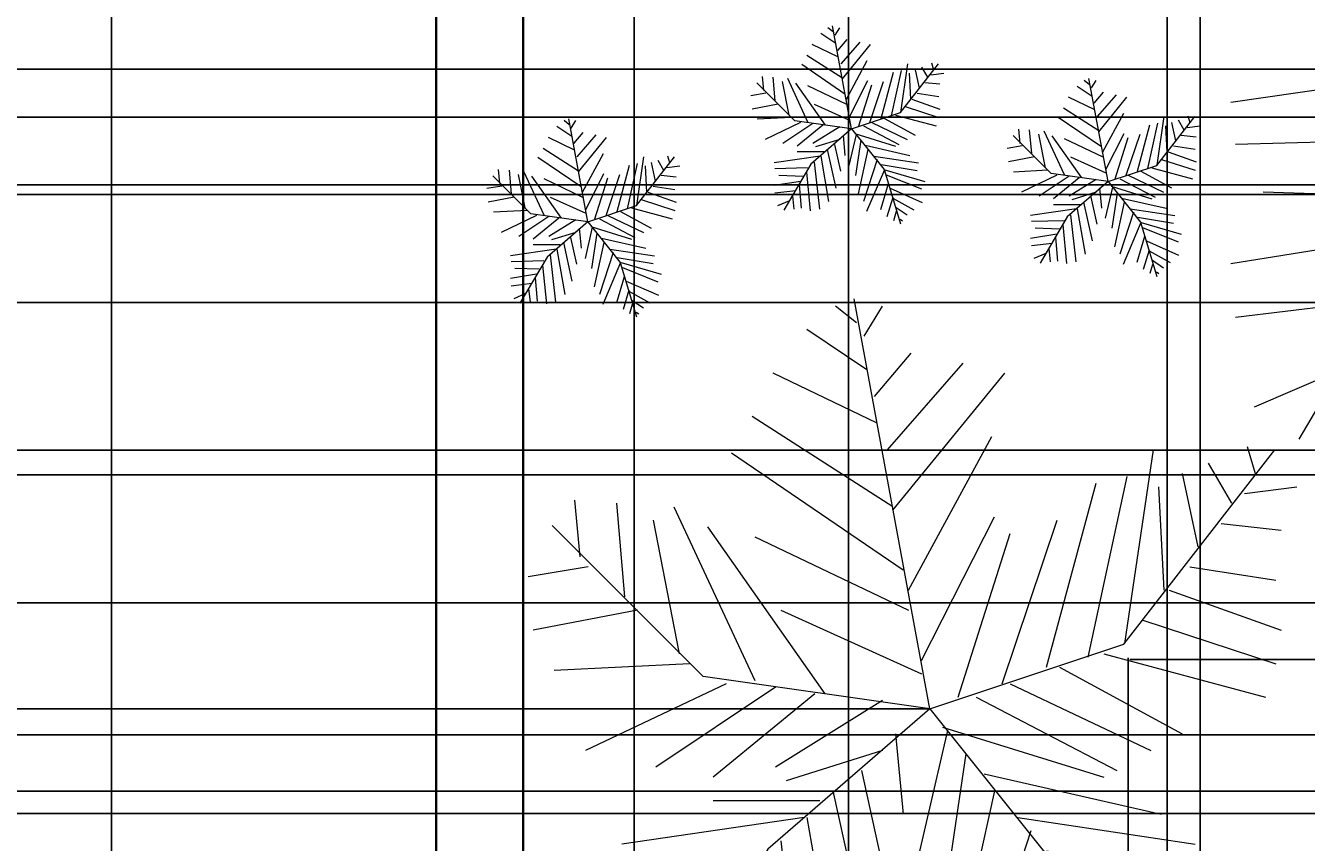
# Model space of a CAD drawing. Units: inches. Extents: x 818 to 1898, y 976 to 2364.
# Tile 58 of 96: x 950 to 1083, y 1873 to 1958. Entities that reach past the tile are written whole.
import ezdxf

# ---------------------------------------------------------------- set-up
doc = ezdxf.new("R2010")
doc.units = ezdxf.units.IN
doc.header["$LTSCALE"] = 5
doc.header["$MEASUREMENT"] = 0
for name, color, linetype, lineweight in [('A-ANNO-DIMS', 2, 'Continuous', 18), ('C-PROP', 7, 'Continuous', 35), ('L-PLNT-BEDS', 94, 'Continuous', 18)]:
    doc.layers.add(name, color=color, linetype=linetype, lineweight=lineweight)
doc.layers.add('L-PLNT', color=116, linetype='Continuous', lineweight=13, true_color=0x136734)
doc.styles.get("Standard").update_dxf_attribs({"font": 'arial.ttf'})
doc.dimstyles.get("Standard").update_dxf_attribs({"dimtxt": 0.18, "dimasz": 0.18, "dimexe": 0.18, "dimexo": 0.0625, "dimgap": 0.09, "dimtad": 0, "dimtih": 1, "dimtoh": 1, "dimdec": 4, "dimzin": 0, "dimdsep": 46, "dimtxsty": 'Standard', "dimcen": 0.09, "dimadec": 0, "dimazin": 0, "dimtfac": 1, "dimtdec": 4, "dimtofl": 0, "dimtmove": 0, "dimatfit": 3, "dimfxl": 1, "dimtolj": 1, "dimtzin": 0, "dimarcsym": 0})

# ---------------------------------------------------------------- blocks, each defined once
blk = doc.blocks.new('SHRUB-ACCENT')
for p, q in [((8.53, 19.84), (7.99, 20.28)), ((10.44, 9.82), (8.47, 20.47)), ((8.74, 19.5), (9.21, 20.28)), ((8.8, 18.63), (7.25, 19.67)), ((9.01, 17.93), (9.96, 19.06)), ((9.35, 16.54), (11.31, 18.8)), ((9.48, 15.07), (5.82, 17.41)), ((9.08, 17.24), (6.37, 18.54)), ((9.48, 14.98), (12.39, 18.54)), ((9.75, 13.42), (5.28, 16.46)), ((9.89, 12.9), (12.06, 16.89)), ((15.49, 11.5), (19.41, 16.55)), ((15.51, 11.51), (16.25, 16.54)), ((17, 15.94), (17.41, 14.03)), ((17.68, 16.2), (18.29, 15.16)), ((18.69, 16.63), (18.9, 15.94)), ((4.55, 10.66), (0.62, 14.58)), ((1.35, 13.77), (1.22, 15.24)), ((2.3, 15.16), (2.51, 12.72)), ((3.25, 14.72), (3.93, 11.25)), ((3.79, 15.07), (5.89, 10.55)), ((10.23, 11.07), (12.12, 14.81)), ((12.33, 10.47), (13.75, 14.72)), ((13.48, 10.9), (14.76, 15.68)), ((14.56, 11.16), (15.58, 15.85)), ((16.39, 15.59), (16.53, 12.9)), ((18.02, 14.63), (19.57, 14.46)), ((18.62, 15.42), (19.98, 15.59)), ((1.56, 13.51), (0, 13.25)), ((7.72, 10.21), (4.67, 14.55)), ((5.89, 14.29), (9.89, 12.38)), ((11.17, 10.12), (12.53, 14.37)), ((17.2, 13.51), (19.44, 13.16)), ((2.84, 12.38), (0.14, 11.86)), ((6.57, 12.38), (10.23, 10.73)), ((15.98, 12.12), (19.44, 10.99)), ((16.66, 12.9), (19.57, 11.86)), ((4.2, 10.99), (0.68, 10.81)), ((10.44, 9.82), (4.55, 10.66)), ((10.44, 9.82), (15.49, 11.5)), ((13.82, 10.9), (17, 9.16)), ((14.97, 11.25), (19.17, 10.12)), ((5.15, 10.47), (1.49, 8.73)), ((6.43, 10.38), (3.32, 8.3)), ((7.45, 10.21), (4.81, 8.04)), ((10.44, 9.82), (6.23, 6.17)), ((9.21, 10.03), (6.43, 8.3)), ((10.44, 9.82), (13.8, 5.61)), ((10.77, 9.34), (14.97, 8.04)), ((11.65, 10.12), (15.31, 8.21)), ((12.53, 10.47), (16.19, 8.73)), ((9.21, 8.73), (6.7, 7.95)), ((8.67, 8.21), (9.28, 5.43)), ((9.55, 9.16), (9.75, 7.08)), ((10.9, 9.25), (10.16, 6.04)), ((11.38, 8.64), (10.84, 5)), ((11.85, 8.12), (16.46, 7.08)), ((7.18, 6.99), (2.44, 6.3)), ((7.59, 7.43), (4.81, 7.43)), ((7.25, 6.99), (8.06, 2.31)), ((7.92, 7.69), (8.8, 3.69)), ((12.12, 7.69), (11.11, 3.09)), ((13.07, 6.65), (11.65, 2.31)), ((12.73, 6.99), (17.34, 6.3)), ((5.89, 5.78), (2.51, 5.69)), ((6.23, 6.17), (3.43, 1.4)), ((5.76, 5.34), (6.16, 1.35)), ((6.57, 6.39), (7.11, 1.52)), ((13.82, 5.6), (11.99, 1.26)), ((13.48, 6.13), (17.2, 5.52)), ((13.8, 5.61), (15.49, 0)), ((13.88, 5.6), (18.02, 4.39)), ((5.15, 4.39), (2.44, 3.95)), ((5.42, 4.91), (2.91, 5)), ((5.01, 4.04), (5.21, 1.61)), ((14.22, 4.13), (13.41, 1.44)), ((14.02, 5.08), (17.68, 3.61)), ((4.67, 3.43), (2.51, 3.17)), ((4.33, 2.91), (4.47, 1.52)), ((14.7, 2.74), (14.09, 0.74)), ((14.43, 3.69), (17.74, 2.22)), ((14.7, 2.65), (16.86, 1.44)), ((4, 2.39), (2.78, 1.87)), ((15.04, 1.7), (16.19, 0.92)), ((15.04, 1.26), (14.76, 0.31)), ((15.44, 0.48), (15.71, 0.31))]:
    blk.add_line(p, q)
blk = doc.blocks.new('PALM-BORDER')
for p, q in [((41.53, 39.05), (33.72, 81.45)), ((33.95, 78.95), (31.8, 80.68)), ((34.76, 77.57), (36.65, 80.68)), ((35.03, 74.11), (28.83, 78.26)), ((35.84, 71.35), (39.61, 75.84)), ((37.18, 65.82), (45, 74.8)), ((36.11, 68.59), (25.33, 73.77)), ((37.72, 59.6), (49.31, 73.77)), ((37.72, 59.95), (23.17, 69.28)), ((39.34, 51.31), (47.96, 67.2)), ((38.8, 53.39), (21.02, 65.48)), ((61.61, 45.75), (77.23, 65.83)), ((61.71, 45.79), (64.67, 65.82)), ((74.37, 66.17), (75.18, 63.4)), ((70.33, 64.44), (72.75, 60.3)), ((53.62, 43.37), (58.74, 62.37)), ((57.93, 44.41), (61.97, 63.06)), ((67.63, 63.4), (69.25, 55.81)), ((65.21, 62.02), (65.75, 51.31)), ((74.1, 61.33), (79.49, 62.02)), ((5.39, 54.77), (4.85, 60.64)), ((9.16, 60.3), (9.97, 50.62)), ((15.09, 59.95), (23.44, 41.99)), ((12.93, 58.57), (15.63, 44.75)), ((40.69, 44.06), (48.23, 58.91)), ((49.04, 41.64), (54.7, 58.57)), ((18.1, 42.4), (2.48, 58.02)), ((30.72, 40.61), (18.59, 57.88)), ((44.46, 40.26), (49.85, 57.19)), ((71.68, 58.22), (77.87, 57.53)), ((23.44, 56.84), (39.34, 49.24)), ((6.2, 53.73), (0, 52.7)), ((68.44, 53.73), (77.33, 52.35)), ((66.29, 51.31), (77.87, 47.17)), ((11.32, 49.24), (0.54, 47.17)), ((26.14, 49.24), (40.69, 42.68)), ((63.59, 48.21), (77.33, 43.71)), ((41.53, 39.05), (61.61, 45.75)), ((16.71, 43.71), (2.69, 43.02)), ((59.55, 44.75), (76.26, 40.26)), ((41.53, 39.05), (18.1, 42.4)), ((54.97, 43.37), (67.63, 36.46)), ((20.48, 41.64), (5.93, 34.73)), ((25.6, 41.3), (13.2, 33.01)), ((49.85, 41.64), (64.4, 34.73)), ((29.64, 40.61), (19.13, 31.97)), ((36.65, 39.91), (25.6, 33.01)), ((46.35, 40.26), (60.9, 32.66)), ((41.53, 39.05), (24.79, 24.55)), ((41.53, 39.05), (54.92, 22.32)), ((42.84, 37.15), (59.55, 31.97)), ((37.99, 36.46), (38.8, 28.17)), ((43.38, 36.81), (40.42, 24.02)), ((36.65, 34.73), (26.68, 31.62)), ((45.27, 34.39), (43.11, 19.88)), ((34.49, 32.66), (36.92, 21.61)), ((47.15, 32.32), (65.48, 28.17)), ((31.53, 30.59), (35.03, 14.7)), ((48.23, 30.59), (44.19, 12.28)), ((30.18, 29.55), (19.13, 29.55)), ((28.56, 27.82), (9.7, 25.06)), ((28.83, 27.82), (32.07, 9.17)), ((50.66, 27.82), (68.98, 25.06)), ((26.14, 25.41), (28.29, 6.06)), ((52, 26.44), (46.35, 9.17)), ((24.79, 24.55), (13.63, 5.58)), ((53.62, 24.37), (68.44, 21.95)), ((23.44, 22.99), (9.97, 22.64)), ((22.9, 21.26), (24.52, 5.37)), ((54.97, 22.3), (47.69, 5.02)), ((54.92, 22.32), (61.61, 0)), ((55.24, 22.3), (71.68, 17.46)), ((21.56, 19.53), (11.59, 19.88)), ((55.78, 20.22), (70.33, 14.35)), ((20.48, 17.46), (9.7, 15.73)), ((19.94, 16.08), (20.75, 6.41)), ((56.59, 16.42), (53.35, 5.72)), ((57.39, 14.7), (70.6, 8.83)), ((18.59, 13.66), (9.97, 12.62)), ((17.24, 11.59), (17.78, 6.06)), ((58.47, 10.9), (56.05, 2.95)), ((15.9, 9.52), (11.05, 7.44)), ((58.47, 10.55), (67.09, 5.72)), ((59.82, 6.75), (64.4, 3.64)), ((59.82, 5.02), (58.74, 1.22)), ((61.44, 1.92), (62.51, 1.22))]:
    blk.add_line(p, q)
blk = doc.blocks.new('PALM-DECK')
for p, q in [((51.03, 49.71), (17.33, 44.77)), ((44.29, 43.85), (24.36, 9.97)), ((41.88, 41.07), (17.81, 40.45)), ((38.51, 34.9), (20.7, 35.52)), ((36.59, 31.2), (17.33, 28.11)), ((33.22, 24.41), (17.81, 22.55)), ((28.4, 17), (19.74, 13.3))]:
    blk.add_line(p, q)
blk = doc.blocks.new('*D29')
at = {"layer": 'A-ANNO-DIMS', "color": 0, "lineweight": -2, "ltscale": 5, "transparency": 16777216}
for p, q in [((1064.31, 1870.24), (1064.31, 1892.19)), ((1064.49, 1892.01), (1134.73, 1892.01)), ((1206.15, 1892.01), (1135.91, 1892.01)), ((1206.33, 1870.24), (1206.33, 1892.19))]:
    blk.add_line(p, q, dxfattribs=at)
at = {"layer": 'A-ANNO-DIMS', "color": 0, "ltscale": 5, "transparency": 16777216}
for points in [[(1064.49, 1892.04), (1064.49, 1891.98), (1064.31, 1892.01)], [(1206.15, 1892.04), (1206.15, 1891.98), (1206.33, 1892.01)]]:
    blk.add_solid(points, dxfattribs=at)
at = {"layer": 'Defpoints', "color": 0, "ltscale": 5, "transparency": 16777216}
for p in [(1206.33, 1892.01), (1064.31, 1870.18), (1206.33, 1870.18)]:
    blk.add_point(p, dxfattribs=at)
at = {"layer": 'A-ANNO-DIMS', "color": 0, "ltscale": 5, "transparency": 16777216, "insert": (1135.32, 1892.01), "char_height": 0.18, "attachment_point": 5}
blk.add_mtext('\\A1;142 TYP.', dxfattribs=at)
blk = doc.blocks.new('*D59')
at = {"layer": 'A-ANNO-DIMS', "color": 0, "lineweight": -2, "ltscale": 5, "transparency": 16777216}
for p, q in [((1251.64, 2300.39), (818.03, 2300.39)), ((818.21, 2300.21), (818.21, 1669.95)), ((818.21, 1039.32), (818.21, 1669.59)), ((896.05, 1039.14), (818.03, 1039.14))]:
    blk.add_line(p, q, dxfattribs=at)
at = {"layer": 'A-ANNO-DIMS', "color": 0, "ltscale": 5, "transparency": 16777216}
for points in [[(818.18, 2300.21), (818.24, 2300.21), (818.21, 2300.39)], [(818.18, 1039.32), (818.24, 1039.32), (818.21, 1039.14)]]:
    blk.add_solid(points, dxfattribs=at)
at = {"layer": 'Defpoints', "color": 0, "ltscale": 5, "transparency": 16777216}
for p in [(818.21, 2300.39), (1251.71, 2300.39), (896.11, 1039.14)]:
    blk.add_point(p, dxfattribs=at)
at = {"layer": 'A-ANNO-DIMS', "color": 0, "ltscale": 5, "transparency": 16777216, "insert": (818.21, 1669.77), "char_height": 0.18, "attachment_point": 5}
blk.add_mtext('\\A1;1261.2', dxfattribs=at)
blk = doc.blocks.new('*D60')
at = {"layer": 'A-ANNO-DIMS', "color": 0, "lineweight": -2, "ltscale": 5, "transparency": 16777216}
for p, q in [((992.66, 2294.22), (818.03, 2294.22)), ((818.21, 2294.04), (818.21, 1748.77)), ((818.21, 1203.14), (818.21, 1748.41)), ((992.66, 1202.96), (818.03, 1202.96))]:
    blk.add_line(p, q, dxfattribs=at)
at = {"layer": 'A-ANNO-DIMS', "color": 0, "ltscale": 5, "transparency": 16777216}
for points in [[(818.18, 2294.04), (818.24, 2294.04), (818.21, 2294.22)], [(818.18, 1203.14), (818.24, 1203.14), (818.21, 1202.96)]]:
    blk.add_solid(points, dxfattribs=at)
at = {"layer": 'Defpoints', "color": 0, "ltscale": 5, "transparency": 16777216}
for p in [(818.21, 2294.22), (992.73, 2294.22), (992.73, 1202.96)]:
    blk.add_point(p, dxfattribs=at)
at = {"layer": 'A-ANNO-DIMS', "color": 0, "ltscale": 5, "transparency": 16777216, "insert": (818.21, 1748.59), "char_height": 0.18, "attachment_point": 5}
blk.add_mtext('\\A1;1091.3', dxfattribs=at)
blk = doc.blocks.new('*D61')
at = {"layer": 'A-ANNO-DIMS', "color": 0, "lineweight": -2, "ltscale": 5, "transparency": 16777216}
for p, q in [((1071.73, 1203.03), (1071.73, 2363.87)), ((1071.91, 2363.69), (1250.94, 2363.69)), ((1430.55, 2363.69), (1251.51, 2363.69)), ((1430.73, 1203.03), (1430.73, 2363.87))]:
    blk.add_line(p, q, dxfattribs=at)
at = {"layer": 'A-ANNO-DIMS', "color": 0, "ltscale": 5, "transparency": 16777216}
for points in [[(1071.91, 2363.72), (1071.91, 2363.66), (1071.73, 2363.69)], [(1430.55, 2363.72), (1430.55, 2363.66), (1430.73, 2363.69)]]:
    blk.add_solid(points, dxfattribs=at)
at = {"layer": 'Defpoints', "color": 0, "ltscale": 5, "transparency": 16777216}
for p in [(1430.73, 2363.69), (1071.73, 1202.96), (1430.73, 1202.96)]:
    blk.add_point(p, dxfattribs=at)
at = {"layer": 'A-ANNO-DIMS', "color": 0, "ltscale": 5, "transparency": 16777216, "insert": (1251.23, 2363.69), "char_height": 0.18, "attachment_point": 5}
blk.add_mtext('\\A1;359', dxfattribs=at)
blk = doc.blocks.new('*D74')
at = {"layer": 'A-ANNO-DIMS', "color": 0, "lineweight": -2, "ltscale": 5, "transparency": 16777216}
for p, q in [((1590.66, 1940.08), (818.03, 1940.08)), ((818.21, 1939.9), (818.21, 1925.76)), ((818.21, 1911.26), (818.21, 1925.4)), ((1590.66, 1911.08), (818.03, 1911.08))]:
    blk.add_line(p, q, dxfattribs=at)
at = {"layer": 'A-ANNO-DIMS', "color": 0, "ltscale": 5, "transparency": 16777216}
for points in [[(818.18, 1939.9), (818.24, 1939.9), (818.21, 1940.08)], [(818.18, 1911.26), (818.24, 1911.26), (818.21, 1911.08)]]:
    blk.add_solid(points, dxfattribs=at)
at = {"layer": 'Defpoints', "color": 0, "ltscale": 5, "transparency": 16777216}
for p in [(818.21, 1940.08), (1590.73, 1940.08), (1590.73, 1911.08)]:
    blk.add_point(p, dxfattribs=at)
at = {"layer": 'A-ANNO-DIMS', "color": 0, "ltscale": 5, "transparency": 16777216, "insert": (818.21, 1925.58), "char_height": 0.18, "attachment_point": 5}
blk.add_mtext('\\A1;29', dxfattribs=at)
blk = doc.blocks.new('*D79')
at = {"layer": 'A-ANNO-DIMS', "color": 0, "lineweight": -2, "ltscale": 5, "transparency": 16777216}
for p, q in [((992.73, 1203.03), (992.73, 2363.87)), ((992.91, 2363.69), (1032.01, 2363.69)), ((1071.55, 2363.69), (1032.44, 2363.69)), ((1071.73, 1203.03), (1071.73, 2363.87))]:
    blk.add_line(p, q, dxfattribs=at)
at = {"layer": 'A-ANNO-DIMS', "color": 0, "ltscale": 5, "transparency": 16777216}
for points in [[(992.91, 2363.72), (992.91, 2363.66), (992.73, 2363.69)], [(1071.55, 2363.72), (1071.55, 2363.66), (1071.73, 2363.69)]]:
    blk.add_solid(points, dxfattribs=at)
at = {"layer": 'Defpoints', "color": 0, "ltscale": 5, "transparency": 16777216}
for p in [(1071.73, 2363.69), (992.73, 1202.96), (1071.73, 1202.96)]:
    blk.add_point(p, dxfattribs=at)
at = {"layer": 'A-ANNO-DIMS', "color": 0, "ltscale": 5, "transparency": 16777216, "insert": (1032.23, 2363.69), "char_height": 0.18, "attachment_point": 5}
blk.add_mtext('\\A1;79', dxfattribs=at)
blk = doc.blocks.new('*D90')
at = {"layer": 'A-ANNO-DIMS', "color": 0, "lineweight": -2, "ltscale": 5, "transparency": 16777216}
for p, q in [((904.95, 1071.12), (904.95, 2363.87)), ((905.13, 2363.69), (931.67, 2363.69)), ((958.99, 2363.69), (932.45, 2363.69)), ((959.17, 1071.12), (959.17, 2363.87))]:
    blk.add_line(p, q, dxfattribs=at)
at = {"layer": 'A-ANNO-DIMS', "color": 0, "ltscale": 5, "transparency": 16777216}
for points in [[(905.13, 2363.72), (905.13, 2363.66), (904.95, 2363.69)], [(958.99, 2363.72), (958.99, 2363.66), (959.17, 2363.69)]]:
    blk.add_solid(points, dxfattribs=at)
at = {"layer": 'Defpoints', "color": 0, "ltscale": 5, "transparency": 16777216}
for p in [(959.17, 2363.69), (904.95, 1071.06), (959.17, 1071.06)]:
    blk.add_point(p, dxfattribs=at)
at = {"layer": 'A-ANNO-DIMS', "color": 0, "ltscale": 5, "transparency": 16777216, "insert": (932.06, 2363.69), "char_height": 0.18, "attachment_point": 5}
blk.add_mtext('\\A1;54.22', dxfattribs=at)
blk = doc.blocks.new('*D91')
at = {"layer": 'A-ANNO-DIMS', "color": 0, "lineweight": -2, "ltscale": 5, "transparency": 16777216}
for p, q in [((959.17, 1071.12), (959.17, 2363.87)), ((959.35, 2363.69), (985.8, 2363.69)), ((1013.04, 2363.69), (986.59, 2363.69)), ((1013.22, 1071.12), (1013.22, 2363.87))]:
    blk.add_line(p, q, dxfattribs=at)
at = {"layer": 'A-ANNO-DIMS', "color": 0, "ltscale": 5, "transparency": 16777216}
for points in [[(959.35, 2363.72), (959.35, 2363.66), (959.17, 2363.69)], [(1013.04, 2363.72), (1013.04, 2363.66), (1013.22, 2363.69)]]:
    blk.add_solid(points, dxfattribs=at)
at = {"layer": 'Defpoints', "color": 0, "ltscale": 5, "transparency": 16777216}
for p in [(1013.22, 2363.69), (959.17, 1071.06), (1013.22, 1071.06)]:
    blk.add_point(p, dxfattribs=at)
at = {"layer": 'A-ANNO-DIMS', "color": 0, "ltscale": 5, "transparency": 16777216, "insert": (986.2, 2363.69), "char_height": 0.18, "attachment_point": 5}
blk.add_mtext('\\A1;54.04', dxfattribs=at)
blk = doc.blocks.new('*D92')
at = {"layer": 'A-ANNO-DIMS', "color": 0, "lineweight": -2, "ltscale": 5, "transparency": 16777216}
for p, q in [((1013.22, 1071.12), (1013.22, 2363.87)), ((1013.4, 2363.69), (1040.38, 2363.69)), ((1068.16, 2363.69), (1041.17, 2363.69)), ((1068.34, 1071.12), (1068.34, 2363.87))]:
    blk.add_line(p, q, dxfattribs=at)
at = {"layer": 'A-ANNO-DIMS', "color": 0, "ltscale": 5, "transparency": 16777216}
for points in [[(1013.4, 2363.72), (1013.4, 2363.66), (1013.22, 2363.69)], [(1068.16, 2363.72), (1068.16, 2363.66), (1068.34, 2363.69)]]:
    blk.add_solid(points, dxfattribs=at)
at = {"layer": 'Defpoints', "color": 0, "ltscale": 5, "transparency": 16777216}
for p in [(1068.34, 2363.69), (1013.22, 1071.06), (1068.34, 1071.06)]:
    blk.add_point(p, dxfattribs=at)
at = {"layer": 'A-ANNO-DIMS', "color": 0, "ltscale": 5, "transparency": 16777216, "insert": (1040.78, 2363.69), "char_height": 0.18, "attachment_point": 5}
blk.add_mtext('\\A1;55.12', dxfattribs=at)
blk = doc.blocks.new('*D93')
at = {"layer": 'A-ANNO-DIMS', "color": 0, "lineweight": -2, "ltscale": 5, "transparency": 16777216}
for p, q in [((1068.34, 1071.12), (1068.34, 2363.87)), ((1068.52, 2363.69), (1094.16, 2363.69)), ((1120.58, 2363.69), (1094.94, 2363.69)), ((1120.76, 1071.12), (1120.76, 2363.87))]:
    blk.add_line(p, q, dxfattribs=at)
at = {"layer": 'A-ANNO-DIMS', "color": 0, "ltscale": 5, "transparency": 16777216}
for points in [[(1068.52, 2363.72), (1068.52, 2363.66), (1068.34, 2363.69)], [(1120.58, 2363.72), (1120.58, 2363.66), (1120.76, 2363.69)]]:
    blk.add_solid(points, dxfattribs=at)
at = {"layer": 'Defpoints', "color": 0, "ltscale": 5, "transparency": 16777216}
for p in [(1120.76, 2363.69), (1068.34, 1071.06), (1120.76, 1071.06)]:
    blk.add_point(p, dxfattribs=at)
at = {"layer": 'A-ANNO-DIMS', "color": 0, "ltscale": 5, "transparency": 16777216, "insert": (1094.55, 2363.69), "char_height": 0.18, "attachment_point": 5}
blk.add_mtext('\\A1;52.42', dxfattribs=at)
blk = doc.blocks.new('*D121')
at = {"layer": 'A-ANNO-DIMS', "color": 0, "lineweight": -2, "ltscale": 5, "transparency": 16777216}
for p, q in [((1766.29, 1884.2), (818.03, 1884.2)), ((818.21, 1884.02), (818.21, 1841.14)), ((818.21, 1797.9), (818.21, 1840.78)), ((1766.29, 1797.72), (818.03, 1797.72))]:
    blk.add_line(p, q, dxfattribs=at)
at = {"layer": 'A-ANNO-DIMS', "color": 0, "ltscale": 5, "transparency": 16777216}
for points in [[(818.18, 1884.02), (818.24, 1884.02), (818.21, 1884.2)], [(818.18, 1797.9), (818.24, 1797.9), (818.21, 1797.72)]]:
    blk.add_solid(points, dxfattribs=at)
at = {"layer": 'Defpoints', "color": 0, "ltscale": 5, "transparency": 16777216}
for p in [(818.21, 1884.2), (1766.35, 1884.2), (1766.35, 1797.72)]:
    blk.add_point(p, dxfattribs=at)
at = {"layer": 'A-ANNO-DIMS', "color": 0, "ltscale": 5, "transparency": 16777216, "insert": (818.21, 1840.96), "char_height": 0.18, "attachment_point": 5}
blk.add_mtext('\\A1;86.49', dxfattribs=at)
blk = doc.blocks.new('*D124')
at = {"layer": 'A-ANNO-DIMS', "color": 0, "lineweight": -2, "ltscale": 5, "transparency": 16777216}
for p, q in [((1131.7, 1974.57), (818.03, 1974.57)), ((818.21, 1974.39), (818.21, 1884.68)), ((818.21, 1794.61), (818.21, 1884.32)), ((1138.44, 1794.43), (818.03, 1794.43))]:
    blk.add_line(p, q, dxfattribs=at)
at = {"layer": 'A-ANNO-DIMS', "color": 0, "ltscale": 5, "transparency": 16777216}
for points in [[(818.18, 1974.39), (818.24, 1974.39), (818.21, 1974.57)], [(818.18, 1794.61), (818.24, 1794.61), (818.21, 1794.43)]]:
    blk.add_solid(points, dxfattribs=at)
at = {"layer": 'Defpoints', "color": 0, "ltscale": 5, "transparency": 16777216}
for p in [(818.21, 1974.57), (1131.77, 1974.57), (1138.5, 1794.43)]:
    blk.add_point(p, dxfattribs=at)
at = {"layer": 'A-ANNO-DIMS', "color": 0, "ltscale": 5, "transparency": 16777216, "insert": (818.21, 1884.5), "char_height": 0.18, "attachment_point": 5}
blk.add_mtext('\\A1;180.14', dxfattribs=at)
blk = doc.blocks.new('*D126')
at = {"layer": 'A-ANNO-DIMS', "color": 0, "lineweight": -2, "ltscale": 5, "transparency": 16777216}
for p, q in [((1035.38, 1252.09), (1035.38, 2363.87)), ((1035.56, 2363.69), (1075.41, 2363.69)), ((1116.01, 2363.69), (1076.16, 2363.69)), ((1116.19, 1236.03), (1116.19, 2363.87))]:
    blk.add_line(p, q, dxfattribs=at)
at = {"layer": 'A-ANNO-DIMS', "color": 0, "ltscale": 5, "transparency": 16777216}
for points in [[(1035.56, 2363.72), (1035.56, 2363.66), (1035.38, 2363.69)], [(1116.01, 2363.72), (1116.01, 2363.66), (1116.19, 2363.69)]]:
    blk.add_solid(points, dxfattribs=at)
at = {"layer": 'Defpoints', "color": 0, "ltscale": 5, "transparency": 16777216}
for p in [(1035.38, 2363.69), (1035.38, 1252.02), (1116.19, 1235.96)]:
    blk.add_point(p, dxfattribs=at)
at = {"layer": 'A-ANNO-DIMS', "color": 0, "ltscale": 5, "transparency": 16777216, "insert": (1075.78, 2363.69), "char_height": 0.18, "attachment_point": 5}
blk.add_mtext('\\A1;80.81', dxfattribs=at)
blk = doc.blocks.new('*D131')
at = {"layer": 'A-ANNO-DIMS', "color": 0, "lineweight": -2, "ltscale": 5, "transparency": 16777216}
for p, q in [((1043.71, 1886.9), (818.03, 1886.9)), ((818.21, 1886.72), (818.21, 1805.95)), ((818.21, 1724.81), (818.21, 1805.58)), ((1044.78, 1724.63), (818.03, 1724.63))]:
    blk.add_line(p, q, dxfattribs=at)
at = {"layer": 'A-ANNO-DIMS', "color": 0, "ltscale": 5, "transparency": 16777216}
for points in [[(818.18, 1886.72), (818.24, 1886.72), (818.21, 1886.9)], [(818.18, 1724.81), (818.24, 1724.81), (818.21, 1724.63)]]:
    blk.add_solid(points, dxfattribs=at)
at = {"layer": 'Defpoints', "color": 0, "ltscale": 5, "transparency": 16777216}
for p in [(818.21, 1886.9), (1043.77, 1886.9), (1044.85, 1724.63)]:
    blk.add_point(p, dxfattribs=at)
at = {"layer": 'A-ANNO-DIMS', "color": 0, "ltscale": 5, "transparency": 16777216, "insert": (818.21, 1805.77), "char_height": 0.18, "attachment_point": 5}
blk.add_mtext('\\A1;162.27', dxfattribs=at)
blk = doc.blocks.new('*D132')
at = {"layer": 'A-ANNO-DIMS', "color": 0, "lineweight": -2, "ltscale": 5, "transparency": 16777216}
for p, q in [((1043.71, 2038.76), (818.03, 2038.76)), ((818.21, 2038.58), (818.21, 1963.01)), ((818.21, 1887.08), (818.21, 1962.65)), ((1043.71, 1886.9), (818.03, 1886.9))]:
    blk.add_line(p, q, dxfattribs=at)
at = {"layer": 'A-ANNO-DIMS', "color": 0, "ltscale": 5, "transparency": 16777216}
for points in [[(818.18, 2038.58), (818.24, 2038.58), (818.21, 2038.76)], [(818.18, 1887.08), (818.24, 1887.08), (818.21, 1886.9)]]:
    blk.add_solid(points, dxfattribs=at)
at = {"layer": 'Defpoints', "color": 0, "ltscale": 5, "transparency": 16777216}
for p in [(818.21, 2038.76), (1043.77, 2038.76), (1043.77, 1886.9)]:
    blk.add_point(p, dxfattribs=at)
at = {"layer": 'A-ANNO-DIMS', "color": 0, "ltscale": 5, "transparency": 16777216, "insert": (818.21, 1962.83), "char_height": 0.18, "attachment_point": 5}
blk.add_mtext('\\A1;151.86', dxfattribs=at)
blk = doc.blocks.new('*D162')
at = {"layer": 'A-ANNO-DIMS', "color": 0, "lineweight": -2, "ltscale": 5, "transparency": 16777216}
for p, q in [((1429.16, 1876.08), (818.03, 1876.08)), ((818.21, 1875.9), (818.21, 1871.76)), ((818.21, 1867.26), (818.21, 1871.4)), ((1429.16, 1867.08), (818.03, 1867.08))]:
    blk.add_line(p, q, dxfattribs=at)
at = {"layer": 'A-ANNO-DIMS', "color": 0, "ltscale": 5, "transparency": 16777216}
for points in [[(818.18, 1875.9), (818.24, 1875.9), (818.21, 1876.08)], [(818.18, 1867.26), (818.24, 1867.26), (818.21, 1867.08)]]:
    blk.add_solid(points, dxfattribs=at)
at = {"layer": 'Defpoints', "color": 0, "ltscale": 5, "transparency": 16777216}
for p in [(1429.23, 1876.08), (818.21, 1867.08), (1429.23, 1867.08)]:
    blk.add_point(p, dxfattribs=at)
at = {"layer": 'A-ANNO-DIMS', "color": 0, "ltscale": 5, "transparency": 16777216, "insert": (818.21, 1871.58), "char_height": 0.18, "attachment_point": 5}
blk.add_mtext('\\A1;9', dxfattribs=at)
blk = doc.blocks.new('*D206')
at = {"layer": 'A-ANNO-DIMS', "color": 0, "lineweight": -2, "ltscale": 5, "transparency": 16777216}
for p, q in [((1590.66, 1911.08), (818.03, 1911.08)), ((818.21, 1910.9), (818.21, 1893.76)), ((818.21, 1876.26), (818.21, 1893.4)), ((1590.66, 1876.08), (818.03, 1876.08))]:
    blk.add_line(p, q, dxfattribs=at)
at = {"layer": 'A-ANNO-DIMS', "color": 0, "ltscale": 5, "transparency": 16777216}
for points in [[(818.18, 1910.9), (818.24, 1910.9), (818.21, 1911.08)], [(818.18, 1876.26), (818.24, 1876.26), (818.21, 1876.08)]]:
    blk.add_solid(points, dxfattribs=at)
at = {"layer": 'Defpoints', "color": 0, "ltscale": 5, "transparency": 16777216}
for p in [(818.21, 1911.08), (1590.73, 1911.08), (1590.73, 1876.08)]:
    blk.add_point(p, dxfattribs=at)
at = {"layer": 'A-ANNO-DIMS', "color": 0, "ltscale": 5, "transparency": 16777216, "insert": (818.21, 1893.58), "char_height": 0.18, "attachment_point": 5}
blk.add_mtext('\\A1;35', dxfattribs=at)
blk = doc.blocks.new('*D211')
at = {"layer": 'A-ANNO-DIMS', "color": 0, "lineweight": -2, "ltscale": 5, "transparency": 16777216}
for p, q in [((1599.66265, 1948.078237), (818.025912, 1948.078237)), ((818.205912, 1947.898237), (818.205912, 1944.758237)), ((818.205912, 1941.258237), (818.205912, 1944.398237)), ((1599.66265, 1941.078237), (818.025912, 1941.078237))]:
    blk.add_line(p, q, dxfattribs=at)
at = {"layer": 'A-ANNO-DIMS', "color": 0, "ltscale": 5, "transparency": 16777216}
for points in [[(818.175912, 1947.898237), (818.235912, 1947.898237), (818.205912, 1948.078237)], [(818.175912, 1941.258237), (818.235912, 1941.258237), (818.205912, 1941.078237)]]:
    blk.add_solid(points, dxfattribs=at)
at = {"layer": 'Defpoints', "color": 0, "ltscale": 5, "transparency": 16777216}
for p in [(818.205912, 1948.078237), (1599.72515, 1948.078237), (1599.72515, 1941.078237)]:
    blk.add_point(p, dxfattribs=at)
at = {"layer": 'A-ANNO-DIMS', "color": 0, "ltscale": 5, "transparency": 16777216, "insert": (818.205912, 1944.578237), "char_height": 0.18, "attachment_point": 5}
blk.add_mtext('\\A1;7', dxfattribs=at)
blk = doc.blocks.new('*D215')
at = {"layer": 'A-ANNO-DIMS', "color": 0, "lineweight": -2, "ltscale": 5, "transparency": 16777216}
for p, q in [((1590.66, 1876.08), (818.03, 1876.08)), ((818.21, 1875.9), (818.21, 1781.76)), ((818.21, 1687.26), (818.21, 1781.4)), ((1511.66, 1687.08), (818.03, 1687.08))]:
    blk.add_line(p, q, dxfattribs=at)
at = {"layer": 'A-ANNO-DIMS', "color": 0, "ltscale": 5, "transparency": 16777216}
for points in [[(818.18, 1875.9), (818.24, 1875.9), (818.21, 1876.08)], [(818.18, 1687.26), (818.24, 1687.26), (818.21, 1687.08)]]:
    blk.add_solid(points, dxfattribs=at)
at = {"layer": 'Defpoints', "color": 0, "ltscale": 5, "transparency": 16777216}
for p in [(818.21, 1876.08), (1590.73, 1876.08), (1511.73, 1687.08)]:
    blk.add_point(p, dxfattribs=at)
at = {"layer": 'A-ANNO-DIMS', "color": 0, "ltscale": 5, "transparency": 16777216, "insert": (818.21, 1781.58), "char_height": 0.18, "attachment_point": 5}
blk.add_mtext('\\A1;189', dxfattribs=at)
blk = doc.blocks.new('*D232')
at = {"layer": 'A-ANNO-DIMS', "color": 0, "lineweight": -2, "ltscale": 5, "transparency": 16777216}
for p, q in [((1303.87, 2008.39), (818.03, 2008.39)), ((818.21, 2008.21), (818.21, 1980.9)), ((818.21, 1953.22), (818.21, 1980.53)), ((1303.87, 1953.04), (818.03, 1953.04))]:
    blk.add_line(p, q, dxfattribs=at)
at = {"layer": 'A-ANNO-DIMS', "color": 0, "ltscale": 5, "transparency": 16777216}
for points in [[(818.18, 2008.21), (818.24, 2008.21), (818.21, 2008.39)], [(818.18, 1953.22), (818.24, 1953.22), (818.21, 1953.04)]]:
    blk.add_solid(points, dxfattribs=at)
at = {"layer": 'Defpoints', "color": 0, "ltscale": 5, "transparency": 16777216}
for p in [(818.21, 2008.39), (1303.93, 2008.39), (1303.93, 1953.04)]:
    blk.add_point(p, dxfattribs=at)
at = {"layer": 'A-ANNO-DIMS', "color": 0, "ltscale": 5, "transparency": 16777216, "insert": (818.21, 1980.72), "char_height": 0.18, "attachment_point": 5}
blk.add_mtext('\\A1;55.35', dxfattribs=at)
blk = doc.blocks.new('*D248')
at = {"layer": 'A-ANNO-DIMS', "color": 0, "lineweight": -2, "ltscale": 5, "transparency": 16777216}
for p, q in [((1258.66, 2019.29), (818.03, 2019.29)), ((818.21, 2019.11), (818.21, 1974.29)), ((818.21, 1929.1), (818.21, 1973.92)), ((1258.66, 1928.92), (818.03, 1928.92))]:
    blk.add_line(p, q, dxfattribs=at)
at = {"layer": 'A-ANNO-DIMS', "color": 0, "ltscale": 5, "transparency": 16777216}
for points in [[(818.18, 2019.11), (818.24, 2019.11), (818.21, 2019.29)], [(818.18, 1929.1), (818.24, 1929.1), (818.21, 1928.92)]]:
    blk.add_solid(points, dxfattribs=at)
at = {"layer": 'Defpoints', "color": 0, "ltscale": 5, "transparency": 16777216}
for p in [(818.21, 2019.29), (1258.73, 2019.29), (1258.73, 1928.92)]:
    blk.add_point(p, dxfattribs=at)
at = {"layer": 'A-ANNO-DIMS', "color": 0, "ltscale": 5, "transparency": 16777216, "insert": (818.21, 1974.1), "char_height": 0.18, "attachment_point": 5}
blk.add_mtext('\\A1;90.37', dxfattribs=at)
blk = doc.blocks.new('*D250')
at = {"layer": 'A-ANNO-DIMS', "color": 0, "lineweight": -2, "ltscale": 5, "transparency": 16777216}
for p, q in [((1250.24, 1913.64), (818.03, 1913.64)), ((818.21, 1913.46), (818.21, 1896.2)), ((818.21, 1878.57), (818.21, 1895.83)), ((1250.24, 1878.39), (818.03, 1878.39))]:
    blk.add_line(p, q, dxfattribs=at)
at = {"layer": 'A-ANNO-DIMS', "color": 0, "ltscale": 5, "transparency": 16777216}
for points in [[(818.18, 1913.46), (818.24, 1913.46), (818.21, 1913.64)], [(818.18, 1878.57), (818.24, 1878.57), (818.21, 1878.39)]]:
    blk.add_solid(points, dxfattribs=at)
at = {"layer": 'Defpoints', "color": 0, "ltscale": 5, "transparency": 16777216}
for p in [(818.21, 1913.64), (1250.3, 1913.64), (1250.3, 1878.39)]:
    blk.add_point(p, dxfattribs=at)
at = {"layer": 'A-ANNO-DIMS', "color": 0, "ltscale": 5, "transparency": 16777216, "insert": (818.21, 1896.02), "char_height": 0.18, "attachment_point": 5}
blk.add_mtext('\\A1;35.25', dxfattribs=at)
blk = doc.blocks.new('*D287')
at = {"layer": 'A-ANNO-DIMS', "color": 0, "lineweight": -2, "ltscale": 5, "transparency": 16777216}
for p, q in [((1303.87, 1953.04), (818.03, 1953.04)), ((818.21, 1952.86), (818.21, 1925.64)), ((818.21, 1898.05), (818.21, 1925.27)), ((1310.96, 1897.87), (818.03, 1897.87))]:
    blk.add_line(p, q, dxfattribs=at)
at = {"layer": 'A-ANNO-DIMS', "color": 0, "ltscale": 5, "transparency": 16777216}
for points in [[(818.18, 1952.86), (818.24, 1952.86), (818.21, 1953.04)], [(818.18, 1898.05), (818.24, 1898.05), (818.21, 1897.87)]]:
    blk.add_solid(points, dxfattribs=at)
at = {"layer": 'Defpoints', "color": 0, "ltscale": 5, "transparency": 16777216}
for p in [(818.21, 1953.04), (1303.93, 1953.04), (1311.03, 1897.87)]:
    blk.add_point(p, dxfattribs=at)
at = {"layer": 'A-ANNO-DIMS', "color": 0, "ltscale": 5, "transparency": 16777216, "insert": (818.21, 1925.45), "char_height": 0.18, "attachment_point": 5}
blk.add_mtext('\\A1;55.17', dxfattribs=at)

msp = doc.modelspace()

# ---------------------------------------------------------------- linework, layer by layer
at = {"layer": 'C-PROP'}
for p, q in [((992.7251, 2294.2171), (992.7251, 1202.9642)), ((1001.7252, 2285.2171), (1001.7252, 1211.9642))]:
    msp.add_line(p, q, dxfattribs=at)
at = {"layer": 'L-PLNT-BEDS'}
msp.add_line((1071.7251, 2214.9709), (1071.7251, 1202.9642), dxfattribs=at)

# ---------------------------------------------------------------- block references
at = {"layer": 'L-PLNT'}
for name, p in [('PALM-DECK', (1057.571, 1904.8049)), ('SHRUB-ACCENT', (1025.2625, 1937.0462)), ('SHRUB-ACCENT', (1051.774, 1931.5924)), ('SHRUB-ACCENT', (997.9712, 1927.4371)), ('PALM-BORDER', (1002.2407, 1847.8507))]:
    msp.add_blockref(name, p, dxfattribs=at)

# ---------------------------------------------------------------- dimensions: what is measured, and where the dimension line sits
at = {"layer": 'A-ANNO-DIMS', "ltscale": 5}
for base, p1, p2, override, picture, middle in [((959.1737, 2363.6929), (904.9504, 1071.0552), (959.1737, 1071.0552), {"dimdec": 2, "dimlfac": 1, "dimrnd": 0, "dimzin": 0, "dimdsep": 46, "dimlunit": 2}, '*D90', (932.062, 2363.6929)), ((1013.2176, 2363.6929), (959.1737, 1071.0552), (1013.2176, 1071.0552), {"dimdec": 2, "dimlfac": 1, "dimrnd": 0, "dimzin": 0, "dimdsep": 46, "dimlunit": 2}, '*D91', (986.1956, 2363.6929)), ((1071.7251, 2363.6929), (992.7251, 1202.9642), (1071.7251, 1202.9642), {"dimdec": 0, "dimlfac": 1, "dimrnd": 0, "dimzin": 0, "dimdsep": 46, "dimlunit": 2}, '*D79', (1032.2251, 2363.6929)), ((1068.3377, 2363.6929), (1013.2176, 1071.0552), (1068.3377, 1071.0552), {"dimdec": 2, "dimlfac": 1, "dimrnd": 0, "dimzin": 0, "dimdsep": 46, "dimlunit": 2}, '*D92', (1040.7776, 2363.6929)), ((1035.3768, 2363.6929), (1116.1882, 1235.9642), (1035.3768, 1252.0242), {"dimdec": 2, "dimlfac": 1, "dimrnd": 0, "dimzin": 0, "dimdsep": 46, "dimlunit": 2}, '*D126', (1075.7825, 2363.6929)), ((1120.7618, 2363.6929), (1068.3377, 1071.0552), (1120.7618, 1071.0552), {"dimdec": 2, "dimlfac": 1, "dimrnd": 0, "dimzin": 0, "dimdsep": 46, "dimlunit": 2}, '*D93', (1094.5497, 2363.6929)), ((1430.7251, 2363.6929), (1071.7251, 1202.9642), (1430.7251, 1202.9642), {"dimdec": 0, "dimlfac": 1, "dimrnd": 0, "dimzin": 0, "dimdsep": 46, "dimlunit": 2}, '*D61', (1251.2251, 2363.6929))]:
    dim = msp.add_linear_dim(base=base, p1=p1, p2=p2, dimstyle='Standard', override=override, dxfattribs=at)
    dim.commit()
    dim.dimension.update_dxf_attribs({"geometry": picture, "text_midpoint": middle})
for base, p1, p2, override, picture, middle in [((818.2059, 2300.3929), (896.1138, 1039.1433), (1251.7057, 2300.3929), {"dimdec": 1, "dimlfac": 1, "dimrnd": 0, "dimzin": 0, "dimdsep": 46, "dimlunit": 2}, '*D59', (818.2059, 1669.7681)), ((818.2059, 2294.2171), (992.7251, 1202.9642), (992.7251, 2294.2171), {"dimdec": 1, "dimlfac": 1, "dimrnd": 0, "dimzin": 0, "dimdsep": 46, "dimlunit": 2}, '*D60', (818.2059, 1748.5907)), ((818.2059, 2038.7583), (1043.7685, 1886.9018), (1043.7685, 2038.7583), {"dimdec": 2, "dimlfac": 1, "dimrnd": 0, "dimzin": 0, "dimdsep": 46, "dimlunit": 2}, '*D132', (818.2059, 1962.83)), ((818.2059, 2019.2871), (1258.7251, 1928.9218), (1258.7251, 2019.2871), {"dimdec": 2, "dimlfac": 1, "dimrnd": 0, "dimzin": 0, "dimdsep": 46, "dimlunit": 2}, '*D248', (818.2059, 1974.1044)), ((818.2059, 2008.3917), (1303.9314, 1953.0408), (1303.9314, 2008.3917), {"dimdec": 2, "dimlfac": 1, "dimrnd": 0, "dimzin": 0, "dimdsep": 46, "dimlunit": 2}, '*D232', (818.2059, 1980.7163)), ((818.2059, 1974.5735), (1138.5041, 1794.4325), (1131.7651, 1974.5735), {"dimdec": 2, "dimlfac": 1, "dimrnd": 0, "dimzin": 0, "dimdsep": 46, "dimlunit": 2}, '*D124', (818.2059, 1884.503)), ((818.2059, 1953.0408), (1311.025, 1897.8663), (1303.9314, 1953.0408), {"dimdec": 2, "dimlfac": 1, "dimrnd": 0, "dimzin": 0, "dimdsep": 46, "dimlunit": 2}, '*D287', (818.2059, 1925.4536)), ((818.2059, 1948.0782), (1599.7251, 1941.0782), (1599.7251, 1948.0782), {"dimdec": 0, "dimlfac": 1, "dimrnd": 0, "dimzin": 0, "dimdsep": 46, "dimlunit": 2}, '*D211', (818.2059, 1944.5782)), ((818.2059, 1940.0782), (1590.7251, 1911.0782), (1590.7251, 1940.0782), {"dimdec": 0, "dimlfac": 1, "dimrnd": 0, "dimzin": 0, "dimdsep": 46, "dimlunit": 2}, '*D74', (818.2059, 1925.5782)), ((818.2059, 1913.6401), (1250.3029, 1878.3919), (1250.3029, 1913.6401), {"dimdec": 2, "dimlfac": 1, "dimrnd": 0, "dimzin": 0, "dimdsep": 46, "dimlunit": 2}, '*D250', (818.2059, 1896.016)), ((818.2059, 1911.0782), (1590.7251, 1876.0782), (1590.7251, 1911.0782), {"dimdec": 0, "dimlfac": 1, "dimrnd": 0, "dimzin": 0, "dimdsep": 46, "dimlunit": 2}, '*D206', (818.2059, 1893.5782)), ((818.2059, 1886.9018), (1044.8463, 1724.63), (1043.7685, 1886.9018), {"dimdec": 2, "dimlfac": 1, "dimrnd": 0, "dimzin": 0, "dimdsep": 46, "dimlunit": 2}, '*D131', (818.2059, 1805.7659)), ((818.2059, 1884.2031), (1766.3524, 1797.7165), (1766.3524, 1884.2031), {"dimdec": 2, "dimlfac": 1, "dimrnd": 0, "dimzin": 0, "dimdsep": 46, "dimlunit": 2}, '*D121', (818.2059, 1840.9598)), ((818.2059, 1876.0782), (1511.7251, 1687.0782), (1590.7251, 1876.0782), {"dimdec": 0, "dimlfac": 1, "dimrnd": 0, "dimzin": 0, "dimdsep": 46, "dimlunit": 2}, '*D215', (818.2059, 1781.5782)), ((818.2059, 1867.0782), (1429.2251, 1876.0782), (1429.2251, 1867.0782), {"dimdec": 0, "dimlfac": 1, "dimrnd": 0, "dimzin": 0, "dimdsep": 46, "dimlunit": 2}, '*D162', (818.2059, 1871.5782))]:
    dim = msp.add_linear_dim(base=base, p1=p1, p2=p2, angle=90, dimstyle='Standard', override=override, dxfattribs=at)
    dim.commit()
    dim.dimension.update_dxf_attribs({"geometry": picture, "text_midpoint": middle})
dim = msp.add_linear_dim(base=(1206.3272, 1892.009), p1=(1064.3101, 1870.1814), p2=(1206.3272, 1870.1814), text='<> TYP.', dimstyle='Standard', override={"dimdec": 0, "dimlfac": 1, "dimrnd": 0, "dimzin": 0, "dimdsep": 46, "dimlunit": 2}, dxfattribs=at)
dim.commit()
dim.dimension.update_dxf_attribs({"geometry": '*D29', "text_midpoint": (1135.3187, 1892.009)})

doc.saveas('drawing.dxf')
